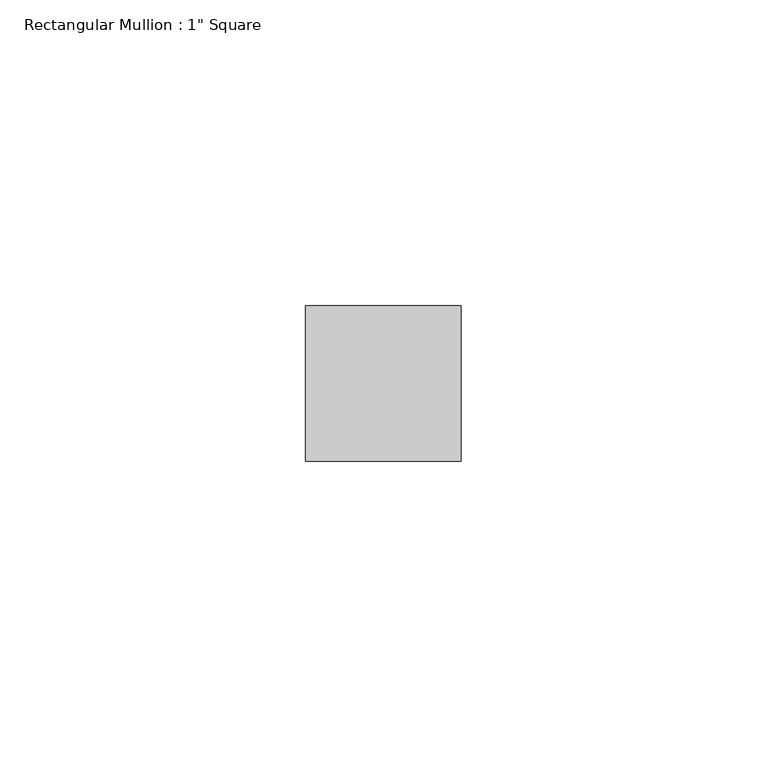
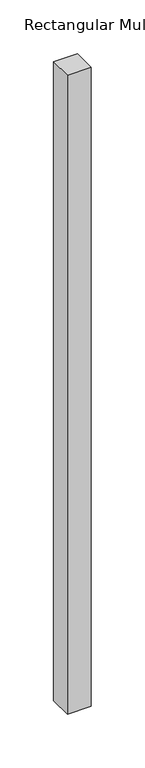
"""IFC4 building model written with IfcOpenShell, lengths in millimetres: member geometry."""

from ifc_helpers import new_model, si_unit, frame, origin, place, context, project, spatial, polyline, outline, extrude, source, transform, mapped, element, save


def member_550490f7(model_context):
    return source(origin(), model_context, "Body", "SweptSolid", [
        extrude(outline(polyline([(12.7, 12.7), (12.7, -12.7), (-12.7, -12.7), (-12.7, 12.7), (12.7, 12.7)])), frame((0.0, 0.0, -723.9), z_axis=(0.0, 0.0, 1.0), x_axis=(1.0, 0.0, 0.0)), (0.0, 0.0, 1.0), 723.9),
    ])


if __name__ == "__main__":
    model = new_model("IFC4")
    model_context = context("Model", 3, world=origin())
    ifc_project = project(units=[si_unit("LENGTHUNIT", "METRE", prefix="MILLI")], contexts=[model_context])
    site = spatial("IfcSite", under=ifc_project)
    building = spatial("IfcBuilding", under=site)
    placement = place(None, origin())
    member_shape = member_550490f7(model_context)
    element("IfcMember", 1, ObjectType="Rectangular Mullion : 1\" Square", at=placement, inside=building, context=model_context, shape_type="MappedRepresentation", body=[
        mapped(member_shape, transform((0.0, 0.0, 0.0), x_axis=(1.0, 0.0, 0.0), y_axis=(0.0, 1.0, 0.0), z_axis=(0.0, 0.0, 1.0))),
    ])
    save(model, "model.ifc")

# Revit data of these elements
# Type "Rectangular Mullion : 1\" Square"
#   built-in parameter 1007304 = 0.0833333 (stored number, unit not read)
#   built-in parameter 1007301 = 0.0416667 (stored number, unit not read)
#   built-in parameter 1007300 = 0.0416667 (stored number, unit not read)
